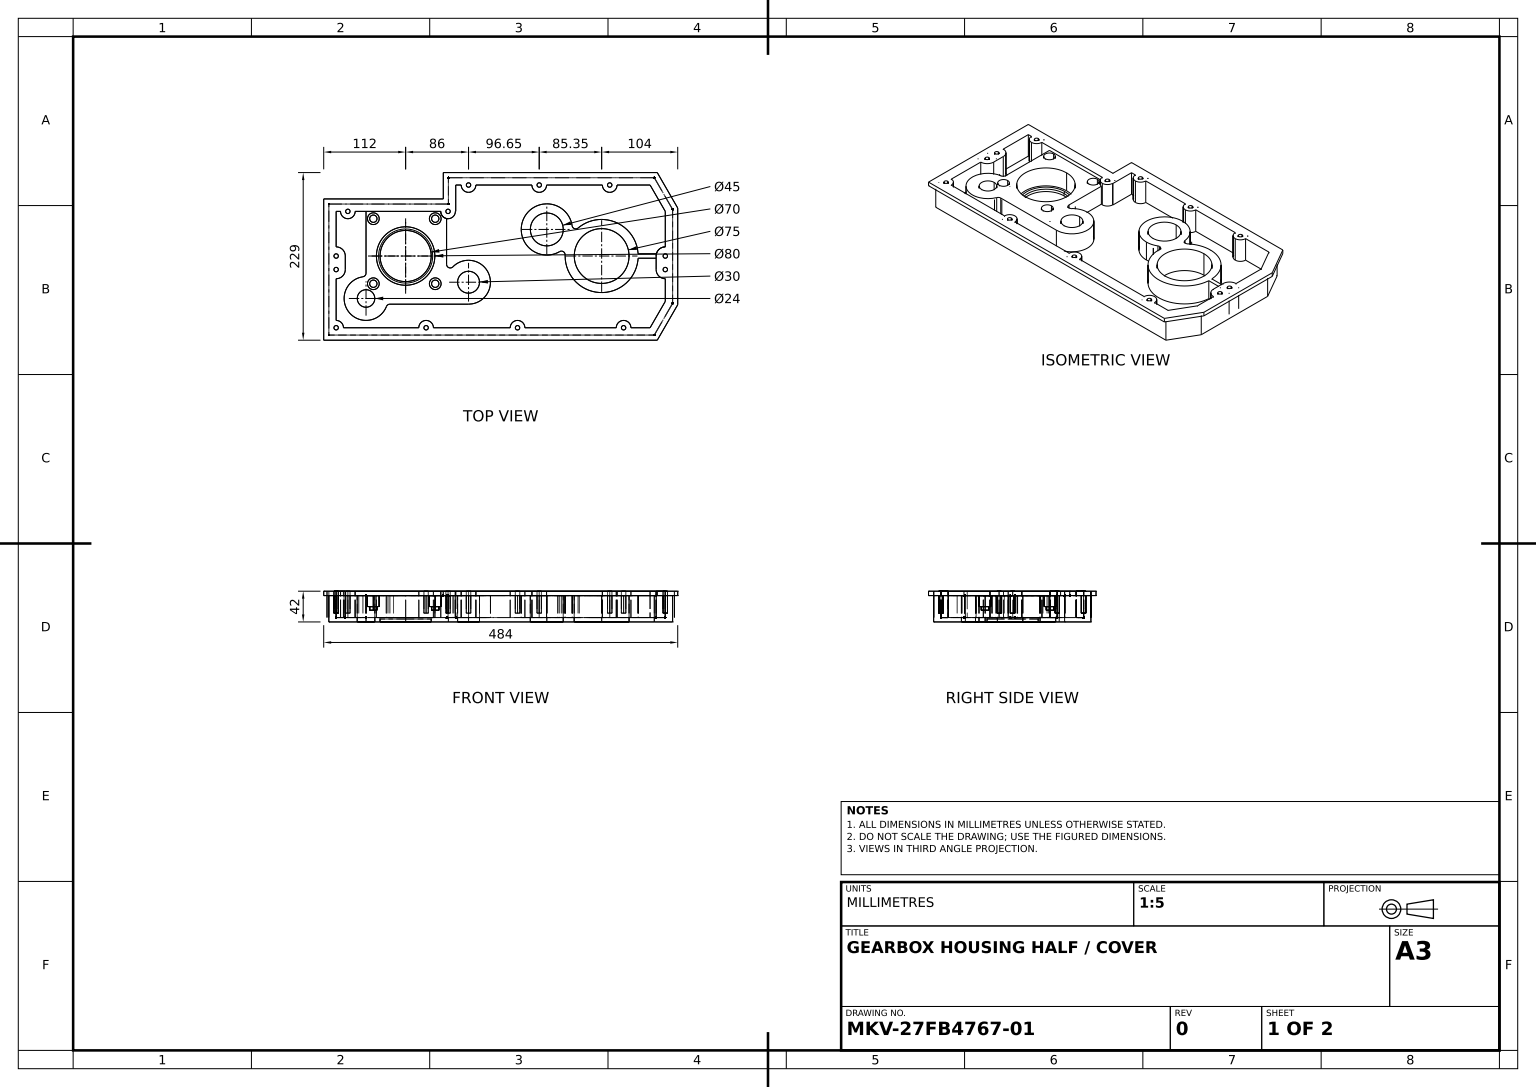
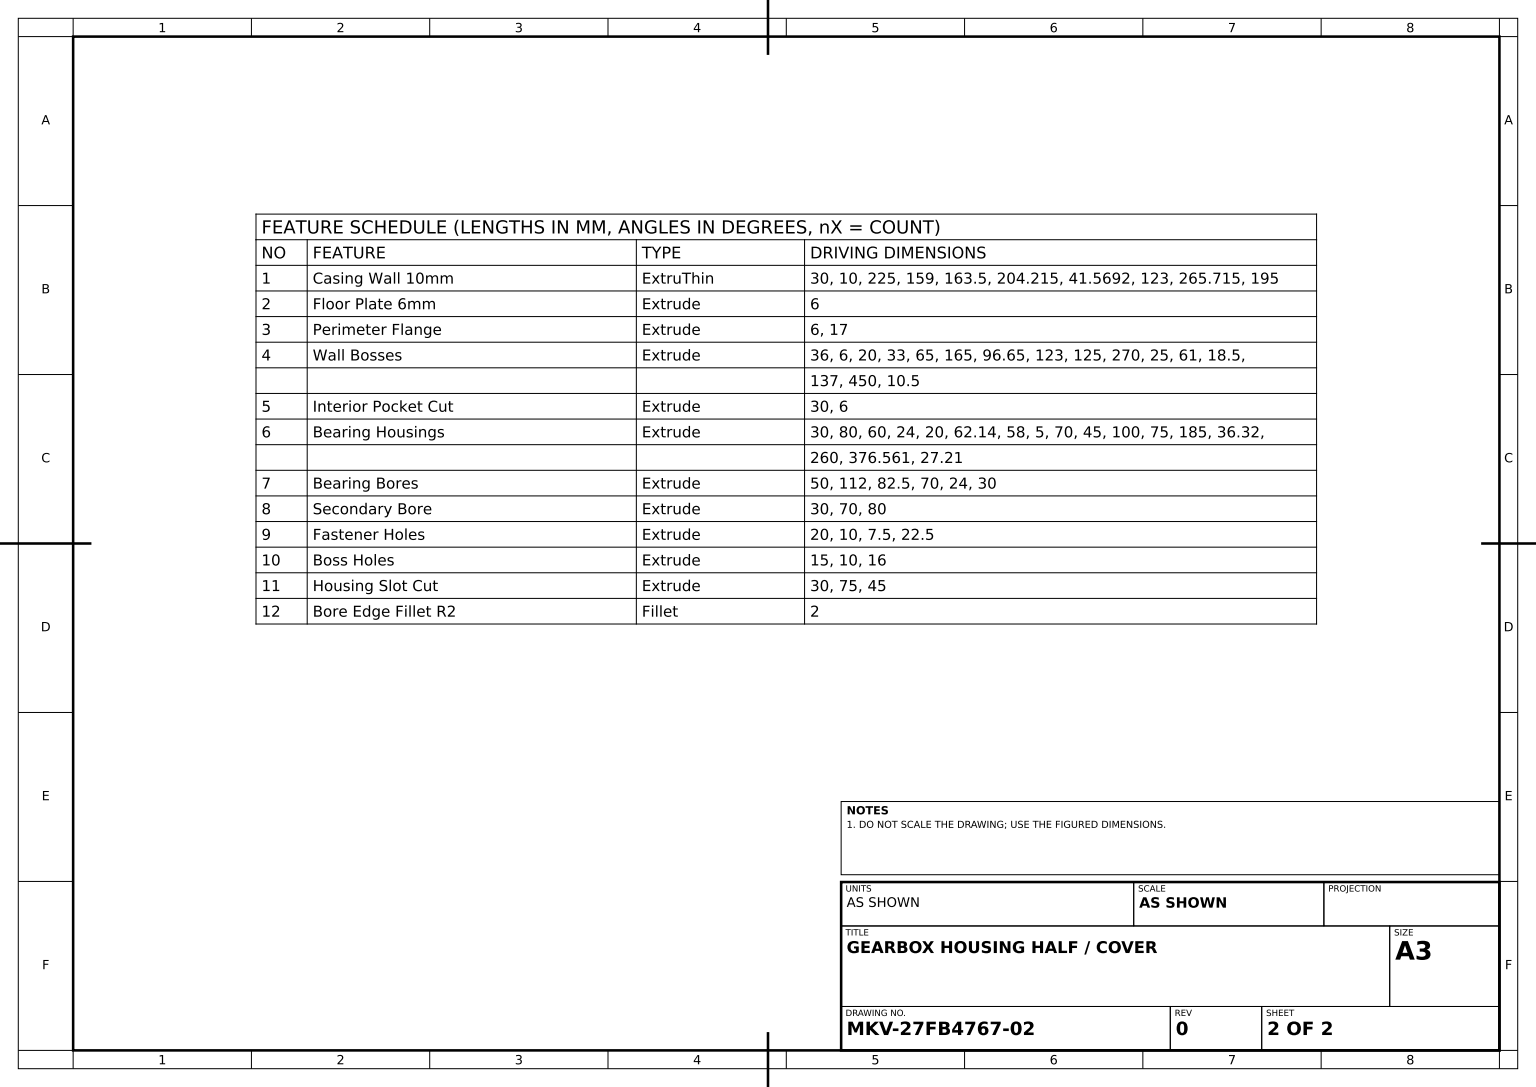
SolidWorks part; units mm, degrees
material "Plain Carbon Steel"
ref_plane "Front Plane" through (0, 0, 0) normal (0, 0, 1) x (1, 0, 0)
ref_plane "Top Plane" through (0, 0, 0) normal (0, 1, 0) x (1, 0, 0)
ref_plane "Right Plane" through (0, 0, 0) normal (1, 0, 0) x (0, 0, -1)
sketch "Casing Outline Sketch" plane through (0, 0, 0) normal (0, 1, 0) x (1, 0, 0)
  line L0 (-225, 0) -> (204.2154, 0)
  line L1 (-225, 0) -> (-225, 159)
  line L2 (-225, 159) -> (-61.5, 159)
  line L3 (-61.5, 159) -> (-61.5, 195)
  line L4 (-61.5, 195) -> (204.2154, 195)
  line L5 (225, 159) -> (225, 36)
  line L8 (225, 159) -> (204.2154, 195)
  line L10 (225, 36) -> (204.2154, 0)
  point P4 (0, 0)
  dimension "D1" = 225
  dimension "D2" = 159
  dimension "D3" = 163.5
  dimension "D4" = 204.2154
  dimension "D5" = 41.5692
  dimension "D6" = 123
  dimension "D7" = 265.7154
  dimension "D8" = 41.5692
  dimension "D9" = 195
  dimension "D10" = 225
extrude "Casing Wall 10mm" add sketch "Casing Outline Sketch" along normal blind 30 thin
sketch "Floor Plate Sketch" plane through (0, 0, 0) normal (0, -1, 0) x (1, 0, 0)
  line L0 (-235, 10) -> (-235, -169)
  line L1 (-235, -169) -> (-71.5, -169)
  line L2 (-71.5, -169) -> (-71.5, -205)
  line L3 (-71.5, -205) -> (209.9889, -205)
  line L4 (209.9889, -205) -> (235, -161.6795)
  line L5 (235, -161.6795) -> (235, -33.3205)
  line L6 (235, -33.3205) -> (209.9889, 10)
  line L7 (209.9889, 10) -> (-235, 10)
extrude "Floor Plate 6mm" add sketch "Floor Plate Sketch" along normal blind 6
sketch "Perimeter Flange Sketch" plane through (0, 30, 0) normal (0, 1, 0) x (1, 0, 0)
  line L1 (-225, 0) -> (-225, 159)
  line L2 (-225, 159) -> (-61.5, 159)
  line L3 (-61.5, 159) -> (-61.5, 195)
  line L4 (204.2154, 195) -> (-61.5, 195) construction
  line L5 (204.2154, 195) -> (-61.5, 195) construction
  line L6 (-61.5, 195) -> (204.2154, 195)
  line L7 (204.2154, 195) -> (225, 159)
  line L8 (225, 159) -> (225, 36)
  line L9 (225, 36) -> (204.2154, 0)
  line L10 (204.2154, 0) -> (-225, 0)
  line L11 (-242, 176) -> (-78.5, 176)
  line L12 (-78.5, 176) -> (-78.5, 212)
  line L13 (-78.5, 212) -> (214.0303, 212)
  line L14 (214.0303, 212) -> (242, 163.5551)
  line L15 (242, 163.5551) -> (242, 31.4449)
  line L16 (242, 31.4449) -> (214.0303, -17)
  line L17 (214.0303, -17) -> (-242, -17)
  line L18 (-242, -17) -> (-242, 176)
  dimension "D1" = 17
extrude "Perimeter Flange" add sketch "Perimeter Flange Sketch" along normal blind 6
sketch "Wall Bosses Sketch" plane through (0, 36, 0) normal (0, 1, 0) x (1, 0, 0)
  line L0 (-61.5, 159) -> (-225, 159) construction
  line L1 (204.2154, 195) -> (-61.5, 195) construction
  line L2 (204.2154, 195) -> (-61.5, 195) construction
  line L3 (-225, 0) -> (204.2154, 0) construction
  line L4 (-242, 176) -> (-242, -17) construction
  line L5 (-225, 110.5) -> (-225, 101)
  line L7 (225, 67) -> (225, 76.5)
  line L9 (159.0303, 195) -> (152.0303, 195)
  line L11 (-61.5, 159) -> (-69, 159)
  line L12 (-222, 0) -> (-215, 0)
  line L13 (-212.5, 98) -> (-212.5, 79.5)
  line L14 (212.5, 98) -> (212.5, 79.5)
  line L15 (-47, 195) -> (-54, 195)
  line L16 (-75, 159) -> (-82, 159)
  line L17 (-199, 159) -> (-206, 159)
  line L18 (-212, 159) -> (-219, 159)
  line L19 (-225, 95) -> (-225, 82.5)
  line L20 (-225, 76.5) -> (-225, 67)
  line L21 (-99, 0) -> (-92, 0)
  line L22 (-112, 0) -> (-105, 0)
  line L23 (-225, 10) -> (-225, 3)
  line L24 (13, 0) -> (20, 0)
  line L25 (26, 0) -> (33, 0)
  line L26 (158, 0) -> (165, 0)
  line L27 (171, 0) -> (178, 0)
  line L28 (225, 101) -> (225, 110.5)
  line L29 (225, 82.5) -> (225, 95)
  line L30 (146.0303, 195) -> (139.0303, 195)
  line L31 (-34, 195) -> (-41, 195)
  line L32 (49.65, 195) -> (42.65, 195)
  line L33 (62.65, 195) -> (55.65, 195)
  circle A0 centre (-225, 0) radius 3
  circle A1 centre (-209, 159) radius 3
  arc A2 (-215, 0) -> (-225, 10) centre (-225, 0) ccw
  arc A3 (-219, 159) -> (-199, 159) centre (-209, 159) ccw
  circle A6 centre (-44, 195) radius 3
  arc A7 (-54, 195) -> (-34, 195) centre (-44, 195) ccw
  circle A8 centre (52.65, 195) radius 3
  arc A9 (42.65, 195) -> (62.65, 195) centre (52.65, 195) ccw
  circle A10 centre (149.0303, 195) radius 3
  arc A11 (139.0303, 195) -> (159.0303, 195) centre (149.0303, 195) ccw
  circle A12 centre (168, 0) radius 3
  arc A13 (178, 0) -> (158, 0) centre (168, 0) ccw
  circle A14 centre (-102, 0) radius 3
  arc A15 (-92, 0) -> (-112, 0) centre (-102, 0) ccw
  circle A18 centre (23, 0) radius 3
  arc A19 (33, 0) -> (13, 0) centre (23, 0) ccw
  circle A20 centre (-225, 98) radius 3
  arc A21 (-212.5, 98) -> (-225, 110.5) centre (-225, 98) ccw
  circle A22 centre (-225, 79.5) radius 3
  arc A23 (-225, 67) -> (-212.5, 79.5) centre (-225, 79.5) ccw
  circle A28 centre (225, 98) radius 3
  circle A30 centre (225, 79.5) radius 3
  arc A31 (212.5, 79.5) -> (225, 67) centre (225, 79.5) ccw
  arc A32 (225, 110.5) -> (212.5, 98) centre (225, 98) ccw
  circle A33 centre (-72, 159) radius 3
  arc A34 (-82, 159) -> (-62, 159) centre (-72, 159) ccw
  line M13 (-61.5, 195) -> (204.2154, 195)
  line M15 (225, 159) -> (225, 36)
  line M17 (204.2154, 0) -> (-225, 0)
  line M18 (-225, 0) -> (-225, 159)
  line M19 (-225, 159) -> (-61.5, 159)
  dimension "D1" = 6
  dimension "D2" = 20
  dimension "D3" = 6
  dimension "D4" = 20
  dimension "D6" = 137
  dimension "D7" = 20
  dimension "D9" = 20
  dimension "D10" = 6
  dimension "D12" = 20
  dimension "D13" = 6
  dimension "D16" = 20
  dimension "D17" = 6
  dimension "D19" = 20
  dimension "D20" = 6
  dimension "D21" = 125
  dimension "D22" = 20
  dimension "D23" = 6
  dimension "D25" = 20
  dimension "D26" = 6
  dimension "D27" = 25
  dimension "D28" = 25
  dimension "D29" = 6
  dimension "D30" = 6
  dimension "D33" = 18.5
  dimension "D34" = 450
  dimension "D35" = 6
  dimension "D36" = 25
  dimension "D37" = 6
  dimension "D8" = 6
  dimension "D5" = 33
  dimension "D11" = 65
  dimension "D14" = 165
  dimension "D15" = 96.65
  dimension "D18" = 123
  dimension "D24" = 270
  dimension "D31" = 61
  dimension "D32" = 18.5
  dimension "D38" = 10.5
extrude "Wall Bosses" add sketch "Wall Bosses Sketch" against normal blind 36 contours A7 A6 M13 | A6 M13 | A6 M13 | A9 A8 M13 | A8 M13 | A8 M13 | A11 A10 M13 | A10 M13 | A10 M13 | A32 L14 A31 A30 A28 M15 | A28 M15 | A28 M15 | A30 M15 | A30 M15 | A3 A1 M19 | A1 M19 | A1 M19 | A33 M19 | A33 M19 | A34 A33 M19 | A20 M18 | A20 M18 | A22 M18 | A22 M18 | A23 L13 A21 A20 A22 M18 | A0 M18 M17 | A0 M17 M18 | A2 A0 M17 M18 | A14 M17 | A14 M17 | A15 A14 M17 | A19 A18 M17 | A18 M17 | A18 M17 | A13 A12 M17 | A12 M17 | A12 M17
sketch "Interior Pocket Sketch" plane through (0, 36, 0) normal (0, 1, 0) x (1, 0, 0)
  circle A0 centre (-209, 159) radius 3
  circle A1 centre (-72, 159) radius 3
  circle A2 centre (-44, 195) radius 3
  circle A3 centre (52.65, 195) radius 3
  circle A4 centre (149.0303, 195) radius 3
  circle A5 centre (225, 98) radius 3
  circle A6 centre (225, 79.5) radius 3
  circle A7 centre (168, 0) radius 3
  circle A8 centre (23, 0) radius 3
  circle A9 centre (-225, 98) radius 3
  circle A10 centre (-225, 79.5) radius 3
  circle A11 centre (-225, 0) radius 3
  circle A12 centre (-102, 0) radius 3
  dimension "D1" = 6
extrude "Interior Pocket Cut" cut sketch "Interior Pocket Sketch" against normal blind 30
sketch "Bearing Housings Sketch" plane through (0, 0, 0) normal (0, 1, 0) x (1, 0, 0)
  line L0 (-102, 3) -> (-102, 0)
  line L2 (187.9099, 95) -> (212.5, 95)
  line L3 (-74, 86.7049) -> (-74, 149.202)
  line L4 (-184.14, 159) -> (-82, 159)
  line L5 (-82, 159) -> (-199, 159) construction
  line L6 (-44, 32.21) -> (-151.5606, 32.21)
  line L7 (-184.14, 74.641) -> (-184.14, 159)
  line L8 (187.9099, 101) -> (212.8653, 101)
  line L9 (212.5, 98) -> (212.5, 95)
  line L10 (212.5, 98) -> (212.5, 79.5) construction
  line L12 (225, 110.5) -> (225, 159) construction
  line L13 (33, 0) -> (158, 0) construction
  circle A0 centre (-122, 98) radius 40
  circle A1 centre (-184.14, 40) radius 12
  arc A2 (-188.4257, 69.6923) -> (-156.2148, 29.0371) centre (-184.14, 40) ccw
  arc A3 (-44, 32.21) -> (-65.4286, 83.2056) centre (-44, 62.21) ccw
  circle A4 centre (-44, 62.21) radius 15
  circle A5 centre (-102, 0) radius 3 construction
  circle A6 centre (-102, 0) radius 3 construction
  arc A7 (-74, 149.202) -> (-82, 159) centre (-72, 159) cw
  arc A8 (-82, 159) -> (-62, 159) centre (-72, 159) ccw construction
  arc A9 (-184.14, 74.641) -> (-188.4257, 69.6923) centre (-189.14, 74.641) cw
  arc A10 (-151.5606, 32.21) -> (-156.2148, 29.0371) centre (-151.5606, 27.21) ccw
  arc A11 (-74, 86.7049) -> (-65.4286, 83.2056) centre (-69, 86.7049) ccw
  arc A12 (88.0237, 99.5401) -> (105.8029, 136.2537) centre (138, 98) ccw
  circle A13 centre (138, 98) radius 37.5
  arc A14 (97.6353, 139.3592) -> (80.5228, 104.0223) centre (63, 134.32) ccw
  circle A15 centre (63, 134.32) radius 22.5
  arc A16 (88.0237, 99.5401) -> (80.5228, 104.0223) centre (83.0261, 99.6941) ccw
  arc A17 (105.8029, 136.2537) -> (97.6353, 139.3592) centre (102.5832, 140.0791) cw
  arc A18 (212.8653, 101) -> (212.5, 98) centre (225, 98) ccw
  arc A19 (225, 110.5) -> (212.5, 98) centre (225, 98) ccw construction
  point P15 (-225, 98)
  point P16 (225, 98)
  point P48 (-225, 95)
  point P49 (225, 95)
  point P50 (-225, 101)
  point P51 (225, 101)
  line M11 (212.5, 79.5) -> (212.5, 98)
  arc M12 (212.5, 98) -> (225, 110.5) centre (225, 98) cw
  arc M24 (-62, 159) -> (-82, 159) centre (-72, 159) cw
  line M25 (-82, 159) -> (-199, 159)
  dimension "D1" = 80
  dimension "D2" = 60
  dimension "D3" = 30
  dimension "D4" = 24
  dimension "D5" = 60
  dimension "D12" = 5
  dimension "D13" = 5
  dimension "D14" = 5
  dimension "D15" = 70
  dimension "D16" = 45
  dimension "D17" = 100
  dimension "D18" = 75
  dimension "D22" = 5
  dimension "D6" = 20
  dimension "D7" = 62.14
  dimension "D8" = 376.5606
  dimension "D9" = 27.21
  dimension "D11" = 58
  dimension "D19" = 185
  dimension "D20" = 36.32
  dimension "D21" = 260
extrude "Bearing Housings" add sketch "Bearing Housings Sketch" along normal blind 30 contours A11 L3 L7 A9 A2 A10 L6 A3 A4 A1 A0 M24 M25 | A12 A17 A14 A16 A15 A13 | A12 L2 L8 M11 M12 | A0
sketch "Bearing Bores Sketch" plane through (0, 30, 0) normal (0, 1, 0) x (1, 0, 0)
  line L0 (-242, 176) -> (-242, -17) construction
  circle A0 centre (-130, 98) radius 35
  circle A1 centre (-184.14, 40) radius 12
  circle A2 centre (-44, 62.21) radius 15
  dimension "D1" = 112
  dimension "D3" = 70
  dimension "D4" = 24
  dimension "D5" = 30
  dimension "D2" = 82.5
extrude "Bearing Bores" cut sketch "Bearing Bores Sketch" against normal blind 50
sketch "Secondary Bore Sketch" plane through (0, 30, 0) normal (0, 1, 0) x (1, 0, 0)
  circle A0 centre (-130, 98) radius 40
  circle A1 centre (-130, 98) radius 35
  dimension "D1" = 70
  dimension "D2" = 80
extrude "Secondary Bore" cut sketch "Secondary Bore Sketch" against normal blind 30
sketch "Fastener Holes Sketch" plane through (0, 30, 0) normal (0, 1, 0) x (1, 0, 0)
  line L0 (-82, 159) -> (-199, 159) construction
  line L1 (-184.14, 74.641) -> (-184.14, 159) construction
  circle A0 centre (-174.14, 149) radius 5
  circle A3 centre (-89.5, 149) radius 5
  circle A4 centre (-89.5, 60.1556) radius 5
  circle A6 centre (-174.14, 60.1556) radius 5
  circle A8 centre (-184.14, 40) radius 12 construction
  dimension "D1" = 10
  dimension "D9" = 10
  dimension "D2" = 10
  dimension "D3" = 7.5
  dimension "D4" = 10
  dimension "D5" = 0
  dimension "D6" = 0
  dimension "D7" = 0
  dimension "D8" = 22.5
extrude "Fastener Holes" cut sketch "Fastener Holes Sketch" against normal blind 20
sketch "Boss Holes Sketch" plane through (0, 30, 0) normal (0, 1, 0) x (1, 0, 0)
  circle A0 centre (-174.14, 149) radius 5
  circle A1 centre (-174.14, 149) radius 8
  circle A2 centre (-89.5, 149) radius 5
  circle A3 centre (-89.5, 149) radius 8
  circle A4 centre (-174.14, 60.1556) radius 5
  circle A5 centre (-174.14, 60.1556) radius 8
  circle A6 centre (-89.5, 60.1556) radius 5
  circle A7 centre (-89.5, 60.1556) radius 8
  dimension "D1" = 10
  dimension "D2" = 16
extrude "Boss Holes" cut sketch "Boss Holes Sketch" against normal blind 15
sketch "Housing Slot Sketch" plane through (0, 0, 0) normal (0, 1, 0) x (1, 0, 0)
  circle A0 centre (63, 134.32) radius 22.5
  circle A1 centre (138, 98) radius 37.5
  dimension "D1" = 75
  dimension "D2" = 45
extrude "Housing Slot Cut" cut sketch "Housing Slot Sketch" against normal blind 30
fillet "Bore Edge Fillet R2" radius 2 1 edges at (-130, 0, -63)
